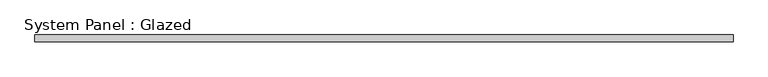
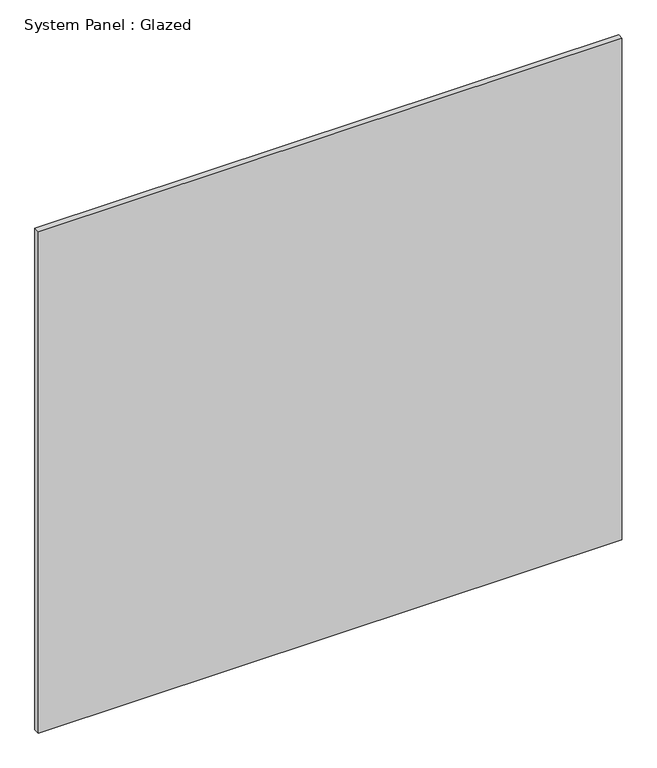
"""IFC4 building model written with IfcOpenShell, lengths in millimetres: plate geometry, System Panel : Glazed."""

from ifc_helpers import new_model, si_unit, origin, origin_with_axes, place, context, project, spatial, polyline, outline, extrude, source, transform, mapped, element, save


def system_panel_glazed_5d90cfdf(model_context):
    return source(origin(), model_context, "Body", "SweptSolid", [
        extrude(outline(polyline([(1272.1166667, 19.05), (-1272.1166667, 19.05), (-1272.1166667, 44.45), (1272.1166667, 44.45), (1272.1166667, 19.05)])), origin_with_axes(), (0.0, 0.0, 1.0), 2311.4),
    ])


if __name__ == "__main__":
    model = new_model("IFC4")
    model_context = context("Model", 3, world=origin())
    ifc_project = project(units=[si_unit("LENGTHUNIT", "METRE", prefix="MILLI")], contexts=[model_context])
    site = spatial("IfcSite", under=ifc_project)
    building = spatial("IfcBuilding", under=site)
    placement = place(None, origin())
    system_panel_glazed_shape = system_panel_glazed_5d90cfdf(model_context)
    element("IfcPlate", 1, ObjectType="System Panel : Glazed", at=placement, inside=building, context=model_context, shape_type="MappedRepresentation", body=[
        mapped(system_panel_glazed_shape, transform((0.0, 0.0, 0.0), x_axis=(1.0, 0.0, 0.0), y_axis=(0.0, 1.0, 0.0), z_axis=(0.0, 0.0, 1.0))),
    ])
    save(model, "model.ifc")

# Revit data of these elements
# Type "System Panel : Glazed"
#   Construction Type Id = "GSP4R"
#   Analytic Construction = "1/8 in Pilkington single glazing"
#   Visual Light Transmittance = 0.9
#   Solar Heat Gain Coefficient = 0.86
#   Heat Transfer Coefficient (U) = 1.18115 BTU/(h·ft²·°F)
# Element 1 (IfcPlate, "System Panel : Glazed")
#   Materials on its faces: "Glass"
# Materials
#   "Glass": class "Glass", colour RGB 0 128 192, transparency 0.75, Description = "Soda Lime Glass", Cost = 0
